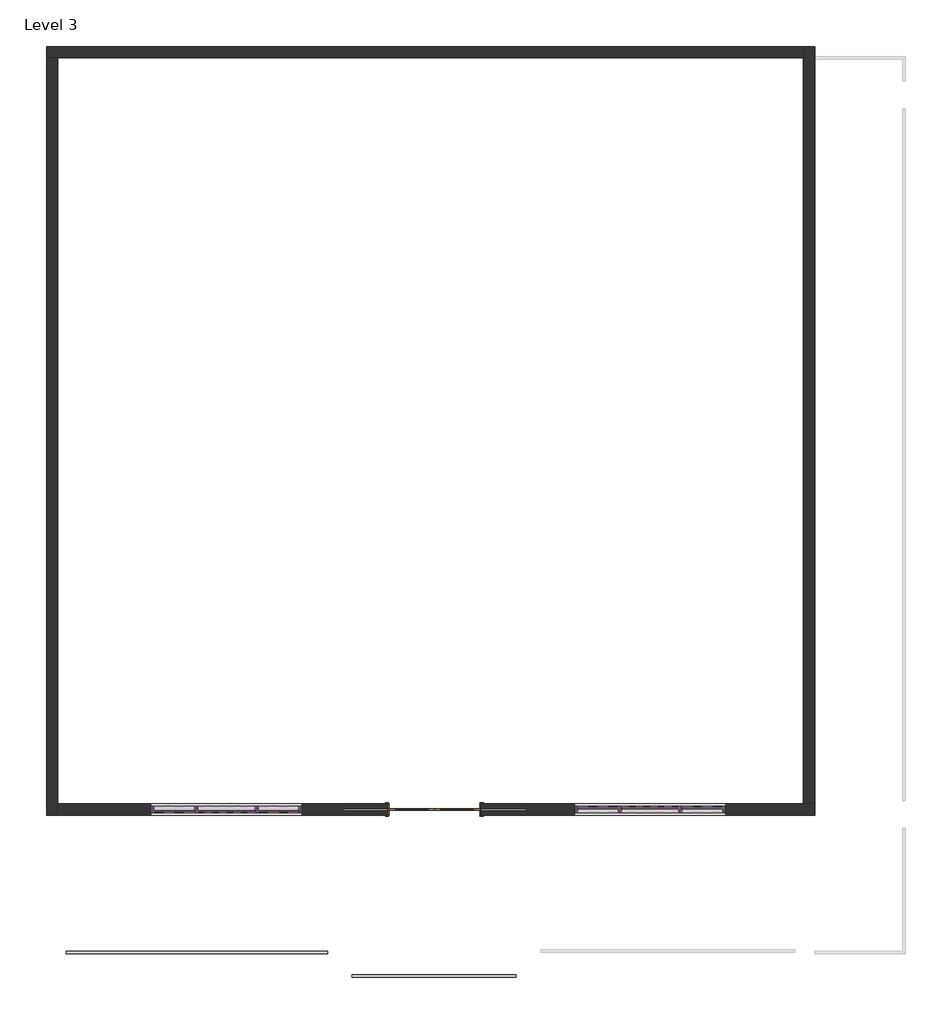
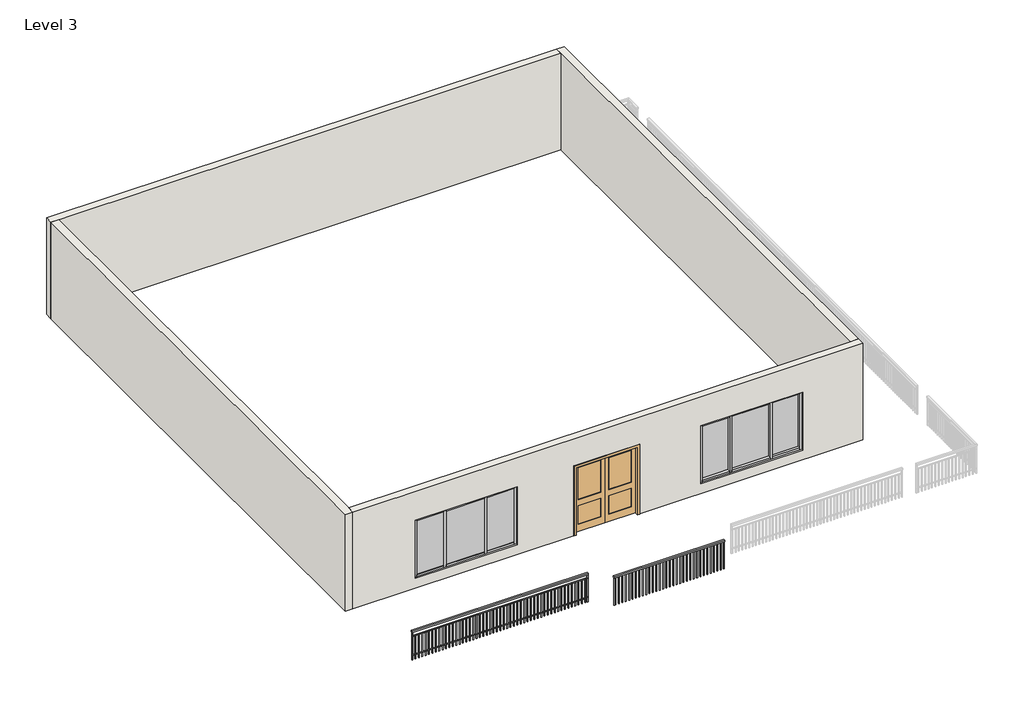
# One storey, part 1 of 4: 20 members, 6 plates, 4 walls, 2 railings, 1 door.
"""IFC4 building model written with IfcOpenShell, lengths in millimetres."""

from ifc_helpers import new_model, si_unit, point, frame, frame_2d, origin, place, context, project, spatial, polyline, circle_curve, trimmed, segment, composite_curve, outline, extrude, faceted_brep, transform, mapped, element, save
from components import door_c75fb906, member_c17f1be2, member_d7472725, member_d60e8053, member_2fae0574, system_panel_glazed_0f3f94b3, system_panel_glazed_6bf442e5

model = new_model("IFC4")

# Units and contexts
model_context = context("Model", 3, world=origin())
ifc_project = project(units=[si_unit("LENGTHUNIT", "METRE", prefix="MILLI")], contexts=[model_context])

# Site, building, storey
site = spatial("IfcSite", under=ifc_project)
building = spatial("IfcBuilding", under=site)
storey = spatial("IfcBuildingStorey", under=building, Name="Level 3", Elevation=3810.0)

# Door
placement = place(None, origin())
door_shape = door_c75fb906(model_context)
element("IfcDoor", 1, ObjectType="Door-Interior-Double-Pocket-2_Panel-Wood : 72\" x 84\"", at=placement, inside=storey, context=model_context, shape_type="MappedRepresentation", body=[
    mapped(door_shape, transform((-962.0249265, -5957.4949916, 3810.0), x_axis=(-1.0, 0.0, 0.0), y_axis=(0.0, -1.0, 0.0), z_axis=(0.0, 0.0, 1.0))),
])

# Members
member_shape = member_c17f1be2(model_context)
element("IfcMember", 2, ObjectType="Rectangular Mullion : 2.5\" x 5\" rectangular", at=placement, inside=storey, context=model_context, shape_type="MappedRepresentation", body=[
    mapped(member_shape, transform((-6613.5249265, -5957.4949916, 5943.6), x_axis=(0.0, 0.0, 1.0), y_axis=(0.0, 1.0, 0.0), z_axis=(-1.0, 0.0, 0.0))),
])
element("IfcMember", 3, ObjectType="Rectangular Mullion : 2.5\" x 5\" rectangular", at=placement, inside=storey, context=model_context, shape_type="MappedRepresentation", body=[
    mapped(member_shape, transform((-4511.6749265, -5957.4949916, 5943.6), x_axis=(0.0, 0.0, 1.0), y_axis=(0.0, 1.0, 0.0), z_axis=(-1.0, 0.0, 0.0))),
])
element("IfcMember", 4, ObjectType="Rectangular Mullion : 2.5\" x 5\" rectangular", at=placement, inside=storey, context=model_context, shape_type="MappedRepresentation", body=[
    mapped(member_shape, transform((4841.8750735, -5957.4949916, 5943.6), x_axis=(0.0, 0.0, 1.0), y_axis=(0.0, -1.0, 0.0), z_axis=(1.0, 0.0, 0.0))),
])
element("IfcMember", 5, ObjectType="Rectangular Mullion : 2.5\" x 5\" rectangular", at=placement, inside=storey, context=model_context, shape_type="MappedRepresentation", body=[
    mapped(member_shape, transform((2740.0250735, -5957.4949916, 5943.6), x_axis=(0.0, 0.0, 1.0), y_axis=(0.0, -1.0, 0.0), z_axis=(1.0, 0.0, 0.0))),
])
element("IfcMember", 6, ObjectType="Rectangular Mullion : 2.5\" x 5\" rectangular", at=placement, inside=storey, context=model_context, shape_type="MappedRepresentation", body=[
    mapped(member_shape, transform((-3692.5249265, -5957.4949916, 4114.8), x_axis=(0.0, 0.0, -1.0), y_axis=(0.0, 1.0, 0.0), z_axis=(1.0, 0.0, 0.0))),
])
element("IfcMember", 7, ObjectType="Rectangular Mullion : 2.5\" x 5\" rectangular", at=placement, inside=storey, context=model_context, shape_type="MappedRepresentation", body=[
    mapped(member_shape, transform((-5794.3749265, -5957.4949916, 4114.8), x_axis=(0.0, 0.0, -1.0), y_axis=(0.0, 1.0, 0.0), z_axis=(1.0, 0.0, 0.0))),
])
element("IfcMember", 8, ObjectType="Rectangular Mullion : 2.5\" x 5\" rectangular", at=placement, inside=storey, context=model_context, shape_type="MappedRepresentation", body=[
    mapped(member_shape, transform((1920.8750735, -5957.4949916, 4114.8), x_axis=(0.0, 0.0, -1.0), y_axis=(0.0, -1.0, 0.0), z_axis=(-1.0, 0.0, 0.0))),
])
element("IfcMember", 9, ObjectType="Rectangular Mullion : 2.5\" x 5\" rectangular", at=placement, inside=storey, context=model_context, shape_type="MappedRepresentation", body=[
    mapped(member_shape, transform((4022.7250735, -5957.4949916, 4114.8), x_axis=(0.0, 0.0, -1.0), y_axis=(0.0, -1.0, 0.0), z_axis=(-1.0, 0.0, 0.0))),
])
member_2_shape = member_d7472725(model_context)
element("IfcMember", 10, ObjectType="Rectangular Mullion : 2.5\" x 5\" rectangular", at=placement, inside=storey, context=model_context, shape_type="MappedRepresentation", body=[
    mapped(member_2_shape, transform((-4575.1749265, -5957.4949916, 4114.8), x_axis=(0.0, 0.0, -1.0), y_axis=(0.0, 1.0, 0.0), z_axis=(1.0, 0.0, 0.0))),
])
element("IfcMember", 11, ObjectType="Rectangular Mullion : 2.5\" x 5\" rectangular", at=placement, inside=storey, context=model_context, shape_type="MappedRepresentation", body=[
    mapped(member_2_shape, transform((2803.5250735, -5957.4949916, 4114.8), x_axis=(0.0, 0.0, -1.0), y_axis=(0.0, -1.0, 0.0), z_axis=(-1.0, 0.0, 0.0))),
])
element("IfcMember", 12, ObjectType="Rectangular Mullion : 2.5\" x 5\" rectangular", at=placement, inside=storey, context=model_context, shape_type="MappedRepresentation", body=[
    mapped(member_2_shape, transform((-5730.8749265, -5957.4949916, 5943.6), x_axis=(0.0, 0.0, 1.0), y_axis=(0.0, 1.0, 0.0), z_axis=(-1.0, 0.0, 0.0))),
])
element("IfcMember", 13, ObjectType="Rectangular Mullion : 2.5\" x 5\" rectangular", at=placement, inside=storey, context=model_context, shape_type="MappedRepresentation", body=[
    mapped(member_2_shape, transform((3959.2250735, -5957.4949916, 5943.6), x_axis=(0.0, 0.0, 1.0), y_axis=(0.0, -1.0, 0.0), z_axis=(1.0, 0.0, 0.0))),
])
member_3_shape = member_d60e8053(model_context)
element("IfcMember", 14, ObjectType="Rectangular Mullion : 2.5\" x 5\" rectangular", at=placement, inside=storey, context=model_context, shape_type="MappedRepresentation", body=[
    mapped(member_3_shape, transform((-5762.6249265, -5957.4949916, 4114.8), x_axis=(-1.0, 0.0, 0.0), y_axis=(0.0, 1.0, 0.0), z_axis=(0.0, 0.0, -1.0))),
])
element("IfcMember", 15, ObjectType="Rectangular Mullion : 2.5\" x 5\" rectangular", at=placement, inside=storey, context=model_context, shape_type="MappedRepresentation", body=[
    mapped(member_3_shape, transform((-4543.4249265, -5957.4949916, 4114.8), x_axis=(-1.0, 0.0, 0.0), y_axis=(0.0, 1.0, 0.0), z_axis=(0.0, 0.0, -1.0))),
])
element("IfcMember", 16, ObjectType="Rectangular Mullion : 2.5\" x 5\" rectangular", at=placement, inside=storey, context=model_context, shape_type="MappedRepresentation", body=[
    mapped(member_3_shape, transform((2771.7750735, -5957.4949916, 4114.8), x_axis=(1.0, 0.0, 0.0), y_axis=(0.0, -1.0, 0.0), z_axis=(0.0, 0.0, -1.0))),
])
element("IfcMember", 17, ObjectType="Rectangular Mullion : 2.5\" x 5\" rectangular", at=placement, inside=storey, context=model_context, shape_type="MappedRepresentation", body=[
    mapped(member_3_shape, transform((3990.9750735, -5957.4949916, 4114.8), x_axis=(1.0, 0.0, 0.0), y_axis=(0.0, -1.0, 0.0), z_axis=(0.0, 0.0, -1.0))),
])
member_4_shape = member_2fae0574(model_context)
element("IfcMember", 18, ObjectType="Rectangular Mullion : 2.5\" x 5\" rectangular", at=placement, inside=storey, context=model_context, shape_type="MappedRepresentation", body=[
    mapped(member_4_shape, transform((-3629.0249265, -5957.4949916, 5943.6), x_axis=(1.0, 0.0, 0.0), y_axis=(0.0, 1.0, 0.0), z_axis=(0.0, 0.0, 1.0))),
])
element("IfcMember", 19, ObjectType="Rectangular Mullion : 2.5\" x 5\" rectangular", at=placement, inside=storey, context=model_context, shape_type="MappedRepresentation", body=[
    mapped(member_4_shape, transform((1857.3750735, -5957.4949916, 5943.6), x_axis=(-1.0, 0.0, 0.0), y_axis=(0.0, -1.0, 0.0), z_axis=(0.0, 0.0, 1.0))),
])
element("IfcMember", 20, ObjectType="Rectangular Mullion : 2.5\" x 5\" rectangular", at=placement, inside=storey, context=model_context, shape_type="MappedRepresentation", body=[
    mapped(member_4_shape, transform((-6677.0249265, -5957.4949916, 4114.8), x_axis=(-1.0, 0.0, 0.0), y_axis=(0.0, 1.0, 0.0), z_axis=(0.0, 0.0, -1.0))),
])
element("IfcMember", 21, ObjectType="Rectangular Mullion : 2.5\" x 5\" rectangular", at=placement, inside=storey, context=model_context, shape_type="MappedRepresentation", body=[
    mapped(member_4_shape, transform((4905.3750735, -5957.4949916, 4114.8), x_axis=(1.0, 0.0, 0.0), y_axis=(0.0, -1.0, 0.0), z_axis=(0.0, 0.0, -1.0))),
])

# Plates
system_panel_glazed_shape = system_panel_glazed_0f3f94b3(model_context)
element("IfcPlate", 22, ObjectType="System Panel : Glazed", at=placement, inside=storey, context=model_context, shape_type="MappedRepresentation", body=[
    mapped(system_panel_glazed_shape, transform((-4102.0999265, -5957.4949916, 4178.3), x_axis=(-1.0, 0.0, 0.0), y_axis=(0.0, -1.0, 0.0), z_axis=(0.0, 0.0, 1.0))),
])
element("IfcPlate", 23, ObjectType="System Panel : Glazed", at=placement, inside=storey, context=model_context, shape_type="MappedRepresentation", body=[
    mapped(system_panel_glazed_shape, transform((2330.4500735, -5957.4949916, 4178.3), x_axis=(1.0, 0.0, 0.0), y_axis=(0.0, 1.0, 0.0), z_axis=(0.0, 0.0, 1.0))),
])
element("IfcPlate", 24, ObjectType="System Panel : Glazed", at=placement, inside=storey, context=model_context, shape_type="MappedRepresentation", body=[
    mapped(system_panel_glazed_shape, transform((-6203.9499265, -5957.4949916, 4178.3), x_axis=(-1.0, 0.0, 0.0), y_axis=(0.0, -1.0, 0.0), z_axis=(0.0, 0.0, 1.0))),
])
element("IfcPlate", 25, ObjectType="System Panel : Glazed", at=placement, inside=storey, context=model_context, shape_type="MappedRepresentation", body=[
    mapped(system_panel_glazed_shape, transform((4432.3000735, -5957.4949916, 4178.3), x_axis=(1.0, 0.0, 0.0), y_axis=(0.0, 1.0, 0.0), z_axis=(0.0, 0.0, 1.0))),
])
system_panel_glazed_2_shape = system_panel_glazed_6bf442e5(model_context)
element("IfcPlate", 26, ObjectType="System Panel : Glazed", at=placement, inside=storey, context=model_context, shape_type="MappedRepresentation", body=[
    mapped(system_panel_glazed_2_shape, transform((-5153.0249265, -5957.4949916, 4178.3), x_axis=(-1.0, 0.0, 0.0), y_axis=(0.0, -1.0, 0.0), z_axis=(0.0, 0.0, 1.0))),
])
element("IfcPlate", 27, ObjectType="System Panel : Glazed", at=placement, inside=storey, context=model_context, shape_type="MappedRepresentation", body=[
    mapped(system_panel_glazed_2_shape, transform((3381.3750735, -5957.4949916, 4178.3), x_axis=(1.0, 0.0, 0.0), y_axis=(0.0, 1.0, 0.0), z_axis=(0.0, 0.0, 1.0))),
])

# Railings
element("IfcRailing", 28, ObjectType="Handrail - Rectangular", at=placement, inside=storey, context=model_context, shape_type="SweptSolid", body=[
    extrude(outline(polyline([(-8376.1341656, -8858.0634361), (-8376.1341656, -8807.2634361), (-3118.3341656, -8807.2634361), (-3118.3341656, -8858.0634361), (-8376.1341656, -8858.0634361)])), frame((0.0, 0.0, 4673.6), z_axis=(0.0, 0.0, 1.0), x_axis=(1.0, 0.0, 0.0)), (0.0, 0.0, 1.0), 50.8),
    extrude(outline(composite_curve([segment(trimmed(circle_curve(frame_2d((-8832.6634361, 4559.3)), 12.7), [point((-8819.9634361, 4559.3))], [point((-8845.3634361, 4559.3))], False, "CARTESIAN"), True, "CONTINUOUS"), segment(trimmed(circle_curve(frame_2d((-8832.6634361, 4559.3)), 12.7), [point((-8845.3634361, 4559.3))], [point((-8819.9634361, 4559.3))], False, "CARTESIAN"), True, "CONTINUOUS")], self_intersect=False)), frame((-8376.1341656, 0.0, 0.0), z_axis=(1.0, 0.0, 0.0), x_axis=(0.0, 1.0, 0.0)), (0.0, 0.0, 1.0), 5257.8),
    extrude(outline(composite_curve([segment(trimmed(circle_curve(frame_2d((-8832.6634361, 3949.7)), 12.7), [point((-8819.9634361, 3949.7))], [point((-8845.3634361, 3949.7))], False, "CARTESIAN"), True, "CONTINUOUS"), segment(trimmed(circle_curve(frame_2d((-8832.6634361, 3949.7)), 12.7), [point((-8845.3634361, 3949.7))], [point((-8819.9634361, 3949.7))], False, "CARTESIAN"), True, "CONTINUOUS")], self_intersect=False)), frame((-8376.1341656, 0.0, 0.0), z_axis=(1.0, 0.0, 0.0), x_axis=(0.0, 1.0, 0.0)), (0.0, 0.0, 1.0), 5257.8),
    extrude(outline(polyline([(-3204.0591656, -8842.1884361), (-3204.0591656, -8823.1384361), (-3185.0091656, -8823.1384361), (-3185.0091656, -8842.1884361), (-3204.0591656, -8842.1884361)])), frame((0.0, 0.0, 3810.0), z_axis=(0.0, 0.0, 1.0), x_axis=(1.0, 0.0, 0.0)), (0.0, 0.0, 1.0), 736.6),
    extrude(outline(polyline([(-3305.6591656, -8842.1884361), (-3305.6591656, -8823.1384361), (-3286.6091656, -8823.1384361), (-3286.6091656, -8842.1884361), (-3305.6591656, -8842.1884361)])), frame((0.0, 0.0, 3810.0), z_axis=(0.0, 0.0, 1.0), x_axis=(1.0, 0.0, 0.0)), (0.0, 0.0, 1.0), 736.6),
    extrude(outline(polyline([(-3407.2591656, -8842.1884361), (-3407.2591656, -8823.1384361), (-3388.2091656, -8823.1384361), (-3388.2091656, -8842.1884361), (-3407.2591656, -8842.1884361)])), frame((0.0, 0.0, 3810.0), z_axis=(0.0, 0.0, 1.0), x_axis=(1.0, 0.0, 0.0)), (0.0, 0.0, 1.0), 736.6),
    extrude(outline(polyline([(-3508.8591656, -8842.1884361), (-3508.8591656, -8823.1384361), (-3489.8091656, -8823.1384361), (-3489.8091656, -8842.1884361), (-3508.8591656, -8842.1884361)])), frame((0.0, 0.0, 3810.0), z_axis=(0.0, 0.0, 1.0), x_axis=(1.0, 0.0, 0.0)), (0.0, 0.0, 1.0), 736.6),
    extrude(outline(polyline([(-3610.4591656, -8842.1884361), (-3610.4591656, -8823.1384361), (-3591.4091656, -8823.1384361), (-3591.4091656, -8842.1884361), (-3610.4591656, -8842.1884361)])), frame((0.0, 0.0, 3810.0), z_axis=(0.0, 0.0, 1.0), x_axis=(1.0, 0.0, 0.0)), (0.0, 0.0, 1.0), 736.6),
    extrude(outline(polyline([(-3712.0591656, -8842.1884361), (-3712.0591656, -8823.1384361), (-3693.0091656, -8823.1384361), (-3693.0091656, -8842.1884361), (-3712.0591656, -8842.1884361)])), frame((0.0, 0.0, 3810.0), z_axis=(0.0, 0.0, 1.0), x_axis=(1.0, 0.0, 0.0)), (0.0, 0.0, 1.0), 736.6),
    extrude(outline(polyline([(-3813.6591656, -8842.1884361), (-3813.6591656, -8823.1384361), (-3794.6091656, -8823.1384361), (-3794.6091656, -8842.1884361), (-3813.6591656, -8842.1884361)])), frame((0.0, 0.0, 3810.0), z_axis=(0.0, 0.0, 1.0), x_axis=(1.0, 0.0, 0.0)), (0.0, 0.0, 1.0), 736.6),
    extrude(outline(polyline([(-3915.2591656, -8842.1884361), (-3915.2591656, -8823.1384361), (-3896.2091656, -8823.1384361), (-3896.2091656, -8842.1884361), (-3915.2591656, -8842.1884361)])), frame((0.0, 0.0, 3810.0), z_axis=(0.0, 0.0, 1.0), x_axis=(1.0, 0.0, 0.0)), (0.0, 0.0, 1.0), 736.6),
    extrude(outline(polyline([(-4016.8591656, -8842.1884361), (-4016.8591656, -8823.1384361), (-3997.8091656, -8823.1384361), (-3997.8091656, -8842.1884361), (-4016.8591656, -8842.1884361)])), frame((0.0, 0.0, 3810.0), z_axis=(0.0, 0.0, 1.0), x_axis=(1.0, 0.0, 0.0)), (0.0, 0.0, 1.0), 736.6),
    extrude(outline(polyline([(-4118.4591656, -8842.1884361), (-4118.4591656, -8823.1384361), (-4099.4091656, -8823.1384361), (-4099.4091656, -8842.1884361), (-4118.4591656, -8842.1884361)])), frame((0.0, 0.0, 3810.0), z_axis=(0.0, 0.0, 1.0), x_axis=(1.0, 0.0, 0.0)), (0.0, 0.0, 1.0), 736.6),
    extrude(outline(polyline([(-4220.0591656, -8842.1884361), (-4220.0591656, -8823.1384361), (-4201.0091656, -8823.1384361), (-4201.0091656, -8842.1884361), (-4220.0591656, -8842.1884361)])), frame((0.0, 0.0, 3810.0), z_axis=(0.0, 0.0, 1.0), x_axis=(1.0, 0.0, 0.0)), (0.0, 0.0, 1.0), 736.6),
    extrude(outline(polyline([(-4321.6591656, -8842.1884361), (-4321.6591656, -8823.1384361), (-4302.6091656, -8823.1384361), (-4302.6091656, -8842.1884361), (-4321.6591656, -8842.1884361)])), frame((0.0, 0.0, 3810.0), z_axis=(0.0, 0.0, 1.0), x_axis=(1.0, 0.0, 0.0)), (0.0, 0.0, 1.0), 736.6),
    extrude(outline(polyline([(-4423.2591656, -8842.1884361), (-4423.2591656, -8823.1384361), (-4404.2091656, -8823.1384361), (-4404.2091656, -8842.1884361), (-4423.2591656, -8842.1884361)])), frame((0.0, 0.0, 3810.0), z_axis=(0.0, 0.0, 1.0), x_axis=(1.0, 0.0, 0.0)), (0.0, 0.0, 1.0), 736.6),
    extrude(outline(polyline([(-4524.8591656, -8842.1884361), (-4524.8591656, -8823.1384361), (-4505.8091656, -8823.1384361), (-4505.8091656, -8842.1884361), (-4524.8591656, -8842.1884361)])), frame((0.0, 0.0, 3810.0), z_axis=(0.0, 0.0, 1.0), x_axis=(1.0, 0.0, 0.0)), (0.0, 0.0, 1.0), 736.6),
    extrude(outline(polyline([(-4626.4591656, -8842.1884361), (-4626.4591656, -8823.1384361), (-4607.4091656, -8823.1384361), (-4607.4091656, -8842.1884361), (-4626.4591656, -8842.1884361)])), frame((0.0, 0.0, 3810.0), z_axis=(0.0, 0.0, 1.0), x_axis=(1.0, 0.0, 0.0)), (0.0, 0.0, 1.0), 736.6),
    extrude(outline(polyline([(-4728.0591656, -8842.1884361), (-4728.0591656, -8823.1384361), (-4709.0091656, -8823.1384361), (-4709.0091656, -8842.1884361), (-4728.0591656, -8842.1884361)])), frame((0.0, 0.0, 3810.0), z_axis=(0.0, 0.0, 1.0), x_axis=(1.0, 0.0, 0.0)), (0.0, 0.0, 1.0), 736.6),
    extrude(outline(polyline([(-4829.6591656, -8842.1884361), (-4829.6591656, -8823.1384361), (-4810.6091656, -8823.1384361), (-4810.6091656, -8842.1884361), (-4829.6591656, -8842.1884361)])), frame((0.0, 0.0, 3810.0), z_axis=(0.0, 0.0, 1.0), x_axis=(1.0, 0.0, 0.0)), (0.0, 0.0, 1.0), 736.6),
    extrude(outline(polyline([(-4931.2591656, -8842.1884361), (-4931.2591656, -8823.1384361), (-4912.2091656, -8823.1384361), (-4912.2091656, -8842.1884361), (-4931.2591656, -8842.1884361)])), frame((0.0, 0.0, 3810.0), z_axis=(0.0, 0.0, 1.0), x_axis=(1.0, 0.0, 0.0)), (0.0, 0.0, 1.0), 736.6),
    extrude(outline(polyline([(-5032.8591656, -8842.1884361), (-5032.8591656, -8823.1384361), (-5013.8091656, -8823.1384361), (-5013.8091656, -8842.1884361), (-5032.8591656, -8842.1884361)])), frame((0.0, 0.0, 3810.0), z_axis=(0.0, 0.0, 1.0), x_axis=(1.0, 0.0, 0.0)), (0.0, 0.0, 1.0), 736.6),
    extrude(outline(polyline([(-5134.4591656, -8842.1884361), (-5134.4591656, -8823.1384361), (-5115.4091656, -8823.1384361), (-5115.4091656, -8842.1884361), (-5134.4591656, -8842.1884361)])), frame((0.0, 0.0, 3810.0), z_axis=(0.0, 0.0, 1.0), x_axis=(1.0, 0.0, 0.0)), (0.0, 0.0, 1.0), 736.6),
    extrude(outline(polyline([(-5236.0591656, -8842.1884361), (-5236.0591656, -8823.1384361), (-5217.0091656, -8823.1384361), (-5217.0091656, -8842.1884361), (-5236.0591656, -8842.1884361)])), frame((0.0, 0.0, 3810.0), z_axis=(0.0, 0.0, 1.0), x_axis=(1.0, 0.0, 0.0)), (0.0, 0.0, 1.0), 736.6),
    extrude(outline(polyline([(-5337.6591656, -8842.1884361), (-5337.6591656, -8823.1384361), (-5318.6091656, -8823.1384361), (-5318.6091656, -8842.1884361), (-5337.6591656, -8842.1884361)])), frame((0.0, 0.0, 3810.0), z_axis=(0.0, 0.0, 1.0), x_axis=(1.0, 0.0, 0.0)), (0.0, 0.0, 1.0), 736.6),
    extrude(outline(polyline([(-5439.2591656, -8842.1884361), (-5439.2591656, -8823.1384361), (-5420.2091656, -8823.1384361), (-5420.2091656, -8842.1884361), (-5439.2591656, -8842.1884361)])), frame((0.0, 0.0, 3810.0), z_axis=(0.0, 0.0, 1.0), x_axis=(1.0, 0.0, 0.0)), (0.0, 0.0, 1.0), 736.6),
    extrude(outline(polyline([(-5540.8591656, -8842.1884361), (-5540.8591656, -8823.1384361), (-5521.8091656, -8823.1384361), (-5521.8091656, -8842.1884361), (-5540.8591656, -8842.1884361)])), frame((0.0, 0.0, 3810.0), z_axis=(0.0, 0.0, 1.0), x_axis=(1.0, 0.0, 0.0)), (0.0, 0.0, 1.0), 736.6),
    extrude(outline(polyline([(-5642.4591656, -8842.1884361), (-5642.4591656, -8823.1384361), (-5623.4091656, -8823.1384361), (-5623.4091656, -8842.1884361), (-5642.4591656, -8842.1884361)])), frame((0.0, 0.0, 3810.0), z_axis=(0.0, 0.0, 1.0), x_axis=(1.0, 0.0, 0.0)), (0.0, 0.0, 1.0), 736.6),
    extrude(outline(polyline([(-5744.0591656, -8842.1884361), (-5744.0591656, -8823.1384361), (-5725.0091656, -8823.1384361), (-5725.0091656, -8842.1884361), (-5744.0591656, -8842.1884361)])), frame((0.0, 0.0, 3810.0), z_axis=(0.0, 0.0, 1.0), x_axis=(1.0, 0.0, 0.0)), (0.0, 0.0, 1.0), 736.6),
    extrude(outline(polyline([(-5845.6591656, -8842.1884361), (-5845.6591656, -8823.1384361), (-5826.6091656, -8823.1384361), (-5826.6091656, -8842.1884361), (-5845.6591656, -8842.1884361)])), frame((0.0, 0.0, 3810.0), z_axis=(0.0, 0.0, 1.0), x_axis=(1.0, 0.0, 0.0)), (0.0, 0.0, 1.0), 736.6),
    extrude(outline(polyline([(-5947.2591656, -8842.1884361), (-5947.2591656, -8823.1384361), (-5928.2091656, -8823.1384361), (-5928.2091656, -8842.1884361), (-5947.2591656, -8842.1884361)])), frame((0.0, 0.0, 3810.0), z_axis=(0.0, 0.0, 1.0), x_axis=(1.0, 0.0, 0.0)), (0.0, 0.0, 1.0), 736.6),
    extrude(outline(polyline([(-6048.8591656, -8842.1884361), (-6048.8591656, -8823.1384361), (-6029.8091656, -8823.1384361), (-6029.8091656, -8842.1884361), (-6048.8591656, -8842.1884361)])), frame((0.0, 0.0, 3810.0), z_axis=(0.0, 0.0, 1.0), x_axis=(1.0, 0.0, 0.0)), (0.0, 0.0, 1.0), 736.6),
    extrude(outline(polyline([(-6150.4591656, -8842.1884361), (-6150.4591656, -8823.1384361), (-6131.4091656, -8823.1384361), (-6131.4091656, -8842.1884361), (-6150.4591656, -8842.1884361)])), frame((0.0, 0.0, 3810.0), z_axis=(0.0, 0.0, 1.0), x_axis=(1.0, 0.0, 0.0)), (0.0, 0.0, 1.0), 736.6),
    extrude(outline(polyline([(-6252.0591656, -8842.1884361), (-6252.0591656, -8823.1384361), (-6233.0091656, -8823.1384361), (-6233.0091656, -8842.1884361), (-6252.0591656, -8842.1884361)])), frame((0.0, 0.0, 3810.0), z_axis=(0.0, 0.0, 1.0), x_axis=(1.0, 0.0, 0.0)), (0.0, 0.0, 1.0), 736.6),
    extrude(outline(polyline([(-6353.6591656, -8842.1884361), (-6353.6591656, -8823.1384361), (-6334.6091656, -8823.1384361), (-6334.6091656, -8842.1884361), (-6353.6591656, -8842.1884361)])), frame((0.0, 0.0, 3810.0), z_axis=(0.0, 0.0, 1.0), x_axis=(1.0, 0.0, 0.0)), (0.0, 0.0, 1.0), 736.6),
    extrude(outline(polyline([(-6455.2591656, -8842.1884361), (-6455.2591656, -8823.1384361), (-6436.2091656, -8823.1384361), (-6436.2091656, -8842.1884361), (-6455.2591656, -8842.1884361)])), frame((0.0, 0.0, 3810.0), z_axis=(0.0, 0.0, 1.0), x_axis=(1.0, 0.0, 0.0)), (0.0, 0.0, 1.0), 736.6),
    extrude(outline(polyline([(-6556.8591656, -8842.1884361), (-6556.8591656, -8823.1384361), (-6537.8091656, -8823.1384361), (-6537.8091656, -8842.1884361), (-6556.8591656, -8842.1884361)])), frame((0.0, 0.0, 3810.0), z_axis=(0.0, 0.0, 1.0), x_axis=(1.0, 0.0, 0.0)), (0.0, 0.0, 1.0), 736.6),
    extrude(outline(polyline([(-6658.4591656, -8842.1884361), (-6658.4591656, -8823.1384361), (-6639.4091656, -8823.1384361), (-6639.4091656, -8842.1884361), (-6658.4591656, -8842.1884361)])), frame((0.0, 0.0, 3810.0), z_axis=(0.0, 0.0, 1.0), x_axis=(1.0, 0.0, 0.0)), (0.0, 0.0, 1.0), 736.6),
    extrude(outline(polyline([(-6760.0591656, -8842.1884361), (-6760.0591656, -8823.1384361), (-6741.0091656, -8823.1384361), (-6741.0091656, -8842.1884361), (-6760.0591656, -8842.1884361)])), frame((0.0, 0.0, 3810.0), z_axis=(0.0, 0.0, 1.0), x_axis=(1.0, 0.0, 0.0)), (0.0, 0.0, 1.0), 736.6),
    extrude(outline(polyline([(-6861.6591656, -8842.1884361), (-6861.6591656, -8823.1384361), (-6842.6091656, -8823.1384361), (-6842.6091656, -8842.1884361), (-6861.6591656, -8842.1884361)])), frame((0.0, 0.0, 3810.0), z_axis=(0.0, 0.0, 1.0), x_axis=(1.0, 0.0, 0.0)), (0.0, 0.0, 1.0), 736.6),
    extrude(outline(polyline([(-6963.2591656, -8842.1884361), (-6963.2591656, -8823.1384361), (-6944.2091656, -8823.1384361), (-6944.2091656, -8842.1884361), (-6963.2591656, -8842.1884361)])), frame((0.0, 0.0, 3810.0), z_axis=(0.0, 0.0, 1.0), x_axis=(1.0, 0.0, 0.0)), (0.0, 0.0, 1.0), 736.6),
    extrude(outline(polyline([(-7064.8591656, -8842.1884361), (-7064.8591656, -8823.1384361), (-7045.8091656, -8823.1384361), (-7045.8091656, -8842.1884361), (-7064.8591656, -8842.1884361)])), frame((0.0, 0.0, 3810.0), z_axis=(0.0, 0.0, 1.0), x_axis=(1.0, 0.0, 0.0)), (0.0, 0.0, 1.0), 736.6),
    extrude(outline(polyline([(-7166.4591656, -8842.1884361), (-7166.4591656, -8823.1384361), (-7147.4091656, -8823.1384361), (-7147.4091656, -8842.1884361), (-7166.4591656, -8842.1884361)])), frame((0.0, 0.0, 3810.0), z_axis=(0.0, 0.0, 1.0), x_axis=(1.0, 0.0, 0.0)), (0.0, 0.0, 1.0), 736.6),
    extrude(outline(polyline([(-7268.0591656, -8842.1884361), (-7268.0591656, -8823.1384361), (-7249.0091656, -8823.1384361), (-7249.0091656, -8842.1884361), (-7268.0591656, -8842.1884361)])), frame((0.0, 0.0, 3810.0), z_axis=(0.0, 0.0, 1.0), x_axis=(1.0, 0.0, 0.0)), (0.0, 0.0, 1.0), 736.6),
    extrude(outline(polyline([(-7369.6591656, -8842.1884361), (-7369.6591656, -8823.1384361), (-7350.6091656, -8823.1384361), (-7350.6091656, -8842.1884361), (-7369.6591656, -8842.1884361)])), frame((0.0, 0.0, 3810.0), z_axis=(0.0, 0.0, 1.0), x_axis=(1.0, 0.0, 0.0)), (0.0, 0.0, 1.0), 736.6),
    extrude(outline(polyline([(-7471.2591656, -8842.1884361), (-7471.2591656, -8823.1384361), (-7452.2091656, -8823.1384361), (-7452.2091656, -8842.1884361), (-7471.2591656, -8842.1884361)])), frame((0.0, 0.0, 3810.0), z_axis=(0.0, 0.0, 1.0), x_axis=(1.0, 0.0, 0.0)), (0.0, 0.0, 1.0), 736.6),
    extrude(outline(polyline([(-7572.8591656, -8842.1884361), (-7572.8591656, -8823.1384361), (-7553.8091656, -8823.1384361), (-7553.8091656, -8842.1884361), (-7572.8591656, -8842.1884361)])), frame((0.0, 0.0, 3810.0), z_axis=(0.0, 0.0, 1.0), x_axis=(1.0, 0.0, 0.0)), (0.0, 0.0, 1.0), 736.6),
    extrude(outline(polyline([(-7674.4591656, -8842.1884361), (-7674.4591656, -8823.1384361), (-7655.4091656, -8823.1384361), (-7655.4091656, -8842.1884361), (-7674.4591656, -8842.1884361)])), frame((0.0, 0.0, 3810.0), z_axis=(0.0, 0.0, 1.0), x_axis=(1.0, 0.0, 0.0)), (0.0, 0.0, 1.0), 736.6),
    extrude(outline(polyline([(-7776.0591656, -8842.1884361), (-7776.0591656, -8823.1384361), (-7757.0091656, -8823.1384361), (-7757.0091656, -8842.1884361), (-7776.0591656, -8842.1884361)])), frame((0.0, 0.0, 3810.0), z_axis=(0.0, 0.0, 1.0), x_axis=(1.0, 0.0, 0.0)), (0.0, 0.0, 1.0), 736.6),
    extrude(outline(polyline([(-7877.6591656, -8842.1884361), (-7877.6591656, -8823.1384361), (-7858.6091656, -8823.1384361), (-7858.6091656, -8842.1884361), (-7877.6591656, -8842.1884361)])), frame((0.0, 0.0, 3810.0), z_axis=(0.0, 0.0, 1.0), x_axis=(1.0, 0.0, 0.0)), (0.0, 0.0, 1.0), 736.6),
    extrude(outline(polyline([(-7979.2591656, -8842.1884361), (-7979.2591656, -8823.1384361), (-7960.2091656, -8823.1384361), (-7960.2091656, -8842.1884361), (-7979.2591656, -8842.1884361)])), frame((0.0, 0.0, 3810.0), z_axis=(0.0, 0.0, 1.0), x_axis=(1.0, 0.0, 0.0)), (0.0, 0.0, 1.0), 736.6),
    extrude(outline(polyline([(-8080.8591656, -8842.1884361), (-8080.8591656, -8823.1384361), (-8061.8091656, -8823.1384361), (-8061.8091656, -8842.1884361), (-8080.8591656, -8842.1884361)])), frame((0.0, 0.0, 3810.0), z_axis=(0.0, 0.0, 1.0), x_axis=(1.0, 0.0, 0.0)), (0.0, 0.0, 1.0), 736.6),
    extrude(outline(polyline([(-8182.4591656, -8842.1884361), (-8182.4591656, -8823.1384361), (-8163.4091656, -8823.1384361), (-8163.4091656, -8842.1884361), (-8182.4591656, -8842.1884361)])), frame((0.0, 0.0, 3810.0), z_axis=(0.0, 0.0, 1.0), x_axis=(1.0, 0.0, 0.0)), (0.0, 0.0, 1.0), 736.6),
    extrude(outline(polyline([(-8284.0591656, -8842.1884361), (-8284.0591656, -8823.1384361), (-8265.0091656, -8823.1384361), (-8265.0091656, -8842.1884361), (-8284.0591656, -8842.1884361)])), frame((0.0, 0.0, 3810.0), z_axis=(0.0, 0.0, 1.0), x_axis=(1.0, 0.0, 0.0)), (0.0, 0.0, 1.0), 736.6),
    extrude(outline(polyline([(-3140.5591656, -8845.3634361), (-3140.5591656, -8819.9634361), (-3115.1591656, -8819.9634361), (-3115.1591656, -8845.3634361), (-3140.5591656, -8845.3634361)])), frame((0.0, 0.0, 3810.0), z_axis=(0.0, 0.0, 1.0), x_axis=(1.0, 0.0, 0.0)), (0.0, 0.0, 1.0), 863.6),
    extrude(outline(polyline([(-8379.3091656, -8845.3634361), (-8379.3091656, -8819.9634361), (-8353.9091656, -8819.9634361), (-8353.9091656, -8845.3634361), (-8379.3091656, -8845.3634361)])), frame((0.0, 0.0, 3810.0), z_axis=(0.0, 0.0, 1.0), x_axis=(1.0, 0.0, 0.0)), (0.0, 0.0, 1.0), 863.6),
])
element("IfcRailing", 29, ObjectType="Handrail - Rectangular 2", at=placement, inside=storey, context=model_context, shape_type="SweptSolid", body=[
    extrude(outline(polyline([(682.1408344, -9284.8949916), (682.1408344, -9335.6949916), (-2619.8591656, -9335.6949916), (-2619.8591656, -9284.8949916), (682.1408344, -9284.8949916)])), frame((0.0, 0.0, 4673.6), z_axis=(0.0, 0.0, 1.0), x_axis=(1.0, 0.0, 0.0)), (0.0, 0.0, 1.0), 50.8),
    extrude(outline(polyline([(-2559.5341656, -9300.7699916), (-2559.5341656, -9319.8199916), (-2578.5841656, -9319.8199916), (-2578.5841656, -9300.7699916), (-2559.5341656, -9300.7699916)])), frame((0.0, 0.0, 3810.0), z_axis=(0.0, 0.0, 1.0), x_axis=(1.0, 0.0, 0.0)), (0.0, 0.0, 1.0), 863.6),
    extrude(outline(polyline([(-2457.9341656, -9300.7699916), (-2457.9341656, -9319.8199916), (-2476.9841656, -9319.8199916), (-2476.9841656, -9300.7699916), (-2457.9341656, -9300.7699916)])), frame((0.0, 0.0, 3810.0), z_axis=(0.0, 0.0, 1.0), x_axis=(1.0, 0.0, 0.0)), (0.0, 0.0, 1.0), 863.6),
    extrude(outline(polyline([(-2356.3341656, -9300.7699916), (-2356.3341656, -9319.8199916), (-2375.3841656, -9319.8199916), (-2375.3841656, -9300.7699916), (-2356.3341656, -9300.7699916)])), frame((0.0, 0.0, 3810.0), z_axis=(0.0, 0.0, 1.0), x_axis=(1.0, 0.0, 0.0)), (0.0, 0.0, 1.0), 863.6),
    extrude(outline(polyline([(-2254.7341656, -9300.7699916), (-2254.7341656, -9319.8199916), (-2273.7841656, -9319.8199916), (-2273.7841656, -9300.7699916), (-2254.7341656, -9300.7699916)])), frame((0.0, 0.0, 3810.0), z_axis=(0.0, 0.0, 1.0), x_axis=(1.0, 0.0, 0.0)), (0.0, 0.0, 1.0), 863.6),
    extrude(outline(polyline([(-2153.1341656, -9300.7699916), (-2153.1341656, -9319.8199916), (-2172.1841656, -9319.8199916), (-2172.1841656, -9300.7699916), (-2153.1341656, -9300.7699916)])), frame((0.0, 0.0, 3810.0), z_axis=(0.0, 0.0, 1.0), x_axis=(1.0, 0.0, 0.0)), (0.0, 0.0, 1.0), 863.6),
    extrude(outline(polyline([(-2051.5341656, -9300.7699916), (-2051.5341656, -9319.8199916), (-2070.5841656, -9319.8199916), (-2070.5841656, -9300.7699916), (-2051.5341656, -9300.7699916)])), frame((0.0, 0.0, 3810.0), z_axis=(0.0, 0.0, 1.0), x_axis=(1.0, 0.0, 0.0)), (0.0, 0.0, 1.0), 863.6),
    extrude(outline(polyline([(-1949.9341656, -9300.7699916), (-1949.9341656, -9319.8199916), (-1968.9841656, -9319.8199916), (-1968.9841656, -9300.7699916), (-1949.9341656, -9300.7699916)])), frame((0.0, 0.0, 3810.0), z_axis=(0.0, 0.0, 1.0), x_axis=(1.0, 0.0, 0.0)), (0.0, 0.0, 1.0), 863.6),
    extrude(outline(polyline([(-1848.3341656, -9300.7699916), (-1848.3341656, -9319.8199916), (-1867.3841656, -9319.8199916), (-1867.3841656, -9300.7699916), (-1848.3341656, -9300.7699916)])), frame((0.0, 0.0, 3810.0), z_axis=(0.0, 0.0, 1.0), x_axis=(1.0, 0.0, 0.0)), (0.0, 0.0, 1.0), 863.6),
    extrude(outline(polyline([(-1746.7341656, -9300.7699916), (-1746.7341656, -9319.8199916), (-1765.7841656, -9319.8199916), (-1765.7841656, -9300.7699916), (-1746.7341656, -9300.7699916)])), frame((0.0, 0.0, 3810.0), z_axis=(0.0, 0.0, 1.0), x_axis=(1.0, 0.0, 0.0)), (0.0, 0.0, 1.0), 863.6),
    extrude(outline(polyline([(-1645.1341656, -9300.7699916), (-1645.1341656, -9319.8199916), (-1664.1841656, -9319.8199916), (-1664.1841656, -9300.7699916), (-1645.1341656, -9300.7699916)])), frame((0.0, 0.0, 3810.0), z_axis=(0.0, 0.0, 1.0), x_axis=(1.0, 0.0, 0.0)), (0.0, 0.0, 1.0), 863.6),
    extrude(outline(polyline([(-1543.5341656, -9300.7699916), (-1543.5341656, -9319.8199916), (-1562.5841656, -9319.8199916), (-1562.5841656, -9300.7699916), (-1543.5341656, -9300.7699916)])), frame((0.0, 0.0, 3810.0), z_axis=(0.0, 0.0, 1.0), x_axis=(1.0, 0.0, 0.0)), (0.0, 0.0, 1.0), 863.6),
    extrude(outline(polyline([(-1441.9341656, -9300.7699916), (-1441.9341656, -9319.8199916), (-1460.9841656, -9319.8199916), (-1460.9841656, -9300.7699916), (-1441.9341656, -9300.7699916)])), frame((0.0, 0.0, 3810.0), z_axis=(0.0, 0.0, 1.0), x_axis=(1.0, 0.0, 0.0)), (0.0, 0.0, 1.0), 863.6),
    extrude(outline(polyline([(-1340.3341656, -9300.7699916), (-1340.3341656, -9319.8199916), (-1359.3841656, -9319.8199916), (-1359.3841656, -9300.7699916), (-1340.3341656, -9300.7699916)])), frame((0.0, 0.0, 3810.0), z_axis=(0.0, 0.0, 1.0), x_axis=(1.0, 0.0, 0.0)), (0.0, 0.0, 1.0), 863.6),
    extrude(outline(polyline([(-1238.7341656, -9300.7699916), (-1238.7341656, -9319.8199916), (-1257.7841656, -9319.8199916), (-1257.7841656, -9300.7699916), (-1238.7341656, -9300.7699916)])), frame((0.0, 0.0, 3810.0), z_axis=(0.0, 0.0, 1.0), x_axis=(1.0, 0.0, 0.0)), (0.0, 0.0, 1.0), 863.6),
    extrude(outline(polyline([(-1137.1341656, -9300.7699916), (-1137.1341656, -9319.8199916), (-1156.1841656, -9319.8199916), (-1156.1841656, -9300.7699916), (-1137.1341656, -9300.7699916)])), frame((0.0, 0.0, 3810.0), z_axis=(0.0, 0.0, 1.0), x_axis=(1.0, 0.0, 0.0)), (0.0, 0.0, 1.0), 863.6),
    extrude(outline(polyline([(-1035.5341656, -9300.7699916), (-1035.5341656, -9319.8199916), (-1054.5841656, -9319.8199916), (-1054.5841656, -9300.7699916), (-1035.5341656, -9300.7699916)])), frame((0.0, 0.0, 3810.0), z_axis=(0.0, 0.0, 1.0), x_axis=(1.0, 0.0, 0.0)), (0.0, 0.0, 1.0), 863.6),
    extrude(outline(polyline([(-933.9341656, -9300.7699916), (-933.9341656, -9319.8199916), (-952.9841656, -9319.8199916), (-952.9841656, -9300.7699916), (-933.9341656, -9300.7699916)])), frame((0.0, 0.0, 3810.0), z_axis=(0.0, 0.0, 1.0), x_axis=(1.0, 0.0, 0.0)), (0.0, 0.0, 1.0), 863.6),
    extrude(outline(polyline([(-832.3341656, -9300.7699916), (-832.3341656, -9319.8199916), (-851.3841656, -9319.8199916), (-851.3841656, -9300.7699916), (-832.3341656, -9300.7699916)])), frame((0.0, 0.0, 3810.0), z_axis=(0.0, 0.0, 1.0), x_axis=(1.0, 0.0, 0.0)), (0.0, 0.0, 1.0), 863.6),
    extrude(outline(polyline([(-730.7341656, -9300.7699916), (-730.7341656, -9319.8199916), (-749.7841656, -9319.8199916), (-749.7841656, -9300.7699916), (-730.7341656, -9300.7699916)])), frame((0.0, 0.0, 3810.0), z_axis=(0.0, 0.0, 1.0), x_axis=(1.0, 0.0, 0.0)), (0.0, 0.0, 1.0), 863.6),
    extrude(outline(polyline([(-629.1341656, -9300.7699916), (-629.1341656, -9319.8199916), (-648.1841656, -9319.8199916), (-648.1841656, -9300.7699916), (-629.1341656, -9300.7699916)])), frame((0.0, 0.0, 3810.0), z_axis=(0.0, 0.0, 1.0), x_axis=(1.0, 0.0, 0.0)), (0.0, 0.0, 1.0), 863.6),
    extrude(outline(polyline([(-527.5341656, -9300.7699916), (-527.5341656, -9319.8199916), (-546.5841656, -9319.8199916), (-546.5841656, -9300.7699916), (-527.5341656, -9300.7699916)])), frame((0.0, 0.0, 3810.0), z_axis=(0.0, 0.0, 1.0), x_axis=(1.0, 0.0, 0.0)), (0.0, 0.0, 1.0), 863.6),
    extrude(outline(polyline([(-425.9341656, -9300.7699916), (-425.9341656, -9319.8199916), (-444.9841656, -9319.8199916), (-444.9841656, -9300.7699916), (-425.9341656, -9300.7699916)])), frame((0.0, 0.0, 3810.0), z_axis=(0.0, 0.0, 1.0), x_axis=(1.0, 0.0, 0.0)), (0.0, 0.0, 1.0), 863.6),
    extrude(outline(polyline([(-324.3341656, -9300.7699916), (-324.3341656, -9319.8199916), (-343.3841656, -9319.8199916), (-343.3841656, -9300.7699916), (-324.3341656, -9300.7699916)])), frame((0.0, 0.0, 3810.0), z_axis=(0.0, 0.0, 1.0), x_axis=(1.0, 0.0, 0.0)), (0.0, 0.0, 1.0), 863.6),
    extrude(outline(polyline([(-222.7341656, -9300.7699916), (-222.7341656, -9319.8199916), (-241.7841656, -9319.8199916), (-241.7841656, -9300.7699916), (-222.7341656, -9300.7699916)])), frame((0.0, 0.0, 3810.0), z_axis=(0.0, 0.0, 1.0), x_axis=(1.0, 0.0, 0.0)), (0.0, 0.0, 1.0), 863.6),
    extrude(outline(polyline([(-121.1341656, -9300.7699916), (-121.1341656, -9319.8199916), (-140.1841656, -9319.8199916), (-140.1841656, -9300.7699916), (-121.1341656, -9300.7699916)])), frame((0.0, 0.0, 3810.0), z_axis=(0.0, 0.0, 1.0), x_axis=(1.0, 0.0, 0.0)), (0.0, 0.0, 1.0), 863.6),
    extrude(outline(polyline([(-19.5341656, -9300.7699916), (-19.5341656, -9319.8199916), (-38.5841656, -9319.8199916), (-38.5841656, -9300.7699916), (-19.5341656, -9300.7699916)])), frame((0.0, 0.0, 3810.0), z_axis=(0.0, 0.0, 1.0), x_axis=(1.0, 0.0, 0.0)), (0.0, 0.0, 1.0), 863.6),
    extrude(outline(polyline([(82.0658344, -9300.7699916), (82.0658344, -9319.8199916), (63.0158344, -9319.8199916), (63.0158344, -9300.7699916), (82.0658344, -9300.7699916)])), frame((0.0, 0.0, 3810.0), z_axis=(0.0, 0.0, 1.0), x_axis=(1.0, 0.0, 0.0)), (0.0, 0.0, 1.0), 863.6),
    extrude(outline(polyline([(183.6658344, -9300.7699916), (183.6658344, -9319.8199916), (164.6158344, -9319.8199916), (164.6158344, -9300.7699916), (183.6658344, -9300.7699916)])), frame((0.0, 0.0, 3810.0), z_axis=(0.0, 0.0, 1.0), x_axis=(1.0, 0.0, 0.0)), (0.0, 0.0, 1.0), 863.6),
    extrude(outline(polyline([(285.2658344, -9300.7699916), (285.2658344, -9319.8199916), (266.2158344, -9319.8199916), (266.2158344, -9300.7699916), (285.2658344, -9300.7699916)])), frame((0.0, 0.0, 3810.0), z_axis=(0.0, 0.0, 1.0), x_axis=(1.0, 0.0, 0.0)), (0.0, 0.0, 1.0), 863.6),
    extrude(outline(polyline([(386.8658344, -9300.7699916), (386.8658344, -9319.8199916), (367.8158344, -9319.8199916), (367.8158344, -9300.7699916), (386.8658344, -9300.7699916)])), frame((0.0, 0.0, 3810.0), z_axis=(0.0, 0.0, 1.0), x_axis=(1.0, 0.0, 0.0)), (0.0, 0.0, 1.0), 863.6),
    extrude(outline(polyline([(488.4658344, -9300.7699916), (488.4658344, -9319.8199916), (469.4158344, -9319.8199916), (469.4158344, -9300.7699916), (488.4658344, -9300.7699916)])), frame((0.0, 0.0, 3810.0), z_axis=(0.0, 0.0, 1.0), x_axis=(1.0, 0.0, 0.0)), (0.0, 0.0, 1.0), 863.6),
    extrude(outline(polyline([(590.0658344, -9300.7699916), (590.0658344, -9319.8199916), (571.0158344, -9319.8199916), (571.0158344, -9300.7699916), (590.0658344, -9300.7699916)])), frame((0.0, 0.0, 3810.0), z_axis=(0.0, 0.0, 1.0), x_axis=(1.0, 0.0, 0.0)), (0.0, 0.0, 1.0), 863.6),
    extrude(outline(polyline([(-2600.8091656, -9300.7699916), (-2600.8091656, -9319.8199916), (-2619.8591656, -9319.8199916), (-2619.8591656, -9300.7699916), (-2600.8091656, -9300.7699916)])), frame((0.0, 0.0, 3810.0), z_axis=(0.0, 0.0, 1.0), x_axis=(1.0, 0.0, 0.0)), (0.0, 0.0, 1.0), 863.6),
    extrude(outline(polyline([(682.1408344, -9300.7699916), (682.1408344, -9319.8199916), (663.0908344, -9319.8199916), (663.0908344, -9300.7699916), (682.1408344, -9300.7699916)])), frame((0.0, 0.0, 3810.0), z_axis=(0.0, 0.0, 1.0), x_axis=(1.0, 0.0, 0.0)), (0.0, 0.0, 1.0), 863.6),
])

# Walls
element("IfcWall", 30, ObjectType="9\" wall", at=placement, inside=storey, context=model_context, shape_type="Brep", body=[
    faceted_brep([(-8772.5249265, 9168.2050084, 3810.0), (-8543.9249265, 9168.2050084, 3810.0), (6467.4750735, 9168.2050084, 3810.0), (6467.4750735, 9168.2050084, 6858.0), (-8543.9249265, 9168.2050084, 6858.0), (-8772.5249265, 9168.2050084, 6858.0), (-8772.5249265, 9396.8050084, 3810.0), (-8772.5249265, 9396.8050084, 6858.0), (6467.4750735, 9396.8050084, 6858.0), (6467.4750735, 9396.8050084, 3810.0)], [[[0, 1, 2, 3, 4, 5]], [[6, 7, 8, 9]], [[2, 1, 0, 6, 9]], [[5, 4, 3, 8, 7]], [[0, 5, 7, 6]], [[3, 2, 9, 8]]]),
])
element("IfcWall", 31, ObjectType="9\" wall", at=placement, inside=storey, context=model_context, shape_type="Brep", body=[
    faceted_brep([(-8543.9249265, -6071.7949916, 3810.0), (-8543.9249265, -5843.1949916, 3810.0), (-8543.9249265, 9168.2050084, 3810.0), (-8543.9249265, 9168.2050084, 6858.0), (-8543.9249265, -5843.1949916, 6858.0), (-8543.9249265, -6071.7949916, 6858.0), (-8772.5249265, -6071.7949916, 3810.0), (-8772.5249265, -6071.7949916, 6858.0), (-8772.5249265, 9168.2050084, 6858.0), (-8772.5249265, 9168.2050084, 3810.0)], [[[0, 1, 2, 3, 4, 5]], [[6, 7, 8, 9]], [[2, 1, 0, 6, 9]], [[5, 4, 3, 8, 7]], [[0, 5, 7, 6]], [[3, 2, 9, 8]]]),
])
element("IfcWall", 32, ObjectType="9\" wall", at=placement, inside=storey, context=model_context, shape_type="Brep", body=[
    faceted_brep([(-8543.9249265, -5843.1949916, 6858.0), (6467.4750735, -5843.1949916, 6858.0), (6696.0750735, -5843.1949916, 6858.0), (6696.0750735, -5843.1949916, 3810.0), (6467.4750735, -5843.1949916, 3810.0), (-22.2249265, -5843.1949916, 3810.0), (-22.2249265, -5843.1949916, 5969.0), (-1901.8249265, -5843.1949916, 5969.0), (-1901.8249265, -5843.1949916, 3810.0), (-8543.9249265, -5843.1949916, 3810.0), (1857.3750735, -5843.1949916, 5943.6), (1857.3750735, -5843.1949916, 4114.8), (4905.3750735, -5843.1949916, 4114.8), (4905.3750735, -5843.1949916, 5943.6), (-3629.0249265, -5843.1949916, 4114.8), (-3629.0249265, -5843.1949916, 5943.6), (-6677.0249265, -5843.1949916, 5943.6), (-6677.0249265, -5843.1949916, 4114.8), (6696.0750735, -6071.7949916, 6858.0), (-8543.9249265, -6071.7949916, 6858.0), (-8543.9249265, -6071.7949916, 3810.0), (-1901.8249265, -6071.7949916, 3810.0), (-1901.8249265, -6071.7949916, 5969.0), (-22.2249265, -6071.7949916, 5969.0), (-22.2249265, -6071.7949916, 3810.0), (6696.0750735, -6071.7949916, 3810.0), (1857.3750735, -6071.7949916, 4114.8), (1857.3750735, -6071.7949916, 5943.6), (4905.3750735, -6071.7949916, 5943.6), (4905.3750735, -6071.7949916, 4114.8), (-3629.0249265, -6071.7949916, 5943.6), (-3629.0249265, -6071.7949916, 4114.8), (-6677.0249265, -6071.7949916, 4114.8), (-6677.0249265, -6071.7949916, 5943.6), (-22.2249265, -5978.1324916, 3810.0), (892.1750735, -5978.1324916, 3810.0), (892.1750735, -5936.8574916, 3810.0), (-22.2249265, -5936.8574916, 3810.0), (-1901.8249265, -5936.8574916, 3810.0), (-2816.2249265, -5936.8574916, 3810.0), (-2816.2249265, -5978.1324916, 3810.0), (-1901.8249265, -5978.1324916, 3810.0), (-2816.2249265, -5978.1324916, 5969.0), (-2816.2249265, -5936.8574916, 5969.0), (-1901.8249265, -5936.8574916, 5969.0), (-22.2249265, -5936.8574916, 5969.0), (892.1750735, -5936.8574916, 5969.0), (892.1750735, -5978.1324916, 5969.0), (-22.2249265, -5978.1324916, 5969.0), (-1901.8249265, -5978.1324916, 5969.0)], [[[0, 1, 2, 3, 4, 5, 6, 7, 8, 9], [10, 11, 12, 13], [14, 15, 16, 17]], [[18, 19, 20, 21, 22, 23, 24, 25], [26, 27, 28, 29], [30, 31, 32, 33]], [[3, 25, 24, 34, 35, 36, 37, 5, 4]], [[20, 9, 8, 38, 39, 40, 41, 21]], [[2, 1, 0, 19, 18]], [[3, 2, 18, 25]], [[0, 9, 20, 19]], [[42, 43, 44, 7, 6, 45, 46, 47, 48, 23, 22, 49]], [[42, 49, 41, 40]], [[49, 22, 21, 41]], [[23, 48, 34, 24]], [[48, 47, 35, 34]], [[47, 46, 36, 35]], [[46, 45, 37, 36]], [[45, 6, 5, 37]], [[7, 44, 38, 8]], [[44, 43, 39, 38]], [[43, 42, 40, 39]], [[10, 27, 26, 11]], [[27, 10, 13, 28]], [[28, 13, 12, 29]], [[11, 26, 29, 12]], [[14, 31, 30, 15]], [[15, 30, 33, 16]], [[16, 33, 32, 17]], [[31, 14, 17, 32]]]),
])
element("IfcWall", 33, ObjectType="9\" wall", at=placement, inside=storey, context=model_context, shape_type="Brep", body=[
    faceted_brep([(6467.4750735, 9396.8050084, 3810.0), (6467.4750735, 9168.2050084, 3810.0), (6467.4750735, -5843.1949916, 3810.0), (6467.4750735, -5843.1949916, 6858.0), (6467.4750735, 9168.2050084, 6858.0), (6467.4750735, 9396.8050084, 6858.0), (6696.0750735, 9396.8050084, 3810.0), (6696.0750735, 9396.8050084, 6858.0), (6696.0750735, -5843.1949916, 6858.0), (6696.0750735, -5843.1949916, 3810.0)], [[[0, 1, 2, 3, 4, 5]], [[6, 7, 8, 9]], [[2, 1, 0, 6, 9]], [[5, 4, 3, 8, 7]], [[0, 5, 7, 6]], [[3, 2, 9, 8]]]),
])

save(model, "model.ifc")

# Revit data of these elements
# Type "Door-Interior-Double-Pocket-2_Panel-Wood : 72\" x 84\""
#   Type Mark = "8"
#   Assembly Code = "C1020300"
#   Analytic Construction = "Wooden"
#   Top Rail = 0' - 4 11/16"
#   Thickness = 0' - 1 3/8"
#   Thermal Resistance (R) = 2.5876 (h·ft²·°F)/BTU
#   Stiles = 0' - 4 3/4"
#   Rough Width = 12' - 2"
#   Rough Height = 7' - 4 1/2"
#   Panel Width = 3' - 0"
#   Lock Rail = 0' - 7 1/2"
#   Location [instance default] = 3' - 1"
#   Height = 7' - 0"
#   Width = 6' - 0"
#   Heat Transfer Coefficient (U) = 0.3865 BTU/(h·ft²·°F)
#   Bottom Rail = 0' - 9 1/8"
#   Panel Open [instance default] = no
#   Trim Material = Cherry
#   Panel Material = door wood colour
#   Frame Material = door wood colour
#   Visual Light Transmittance = 0
#   Solar Heat Gain Coefficient = 0
#   Wall Closure = (empty or 0)
#   Function = (empty or 0)
# Type "Rectangular Mullion : 2.5\" x 5\" rectangular"
#   built-in parameter 1007304 = 0.416667 (stored number, unit not read)
#   built-in parameter 1007301 = 0.104167 (stored number, unit not read)
#   built-in parameter 1007300 = 0.104167 (stored number, unit not read)
# Type "System Panel : Glazed"
#   Construction Type Id = "GSP4R"
#   Analytic Construction = "1/8 in Pilkington single glazing"
#   Visual Light Transmittance = 0.9
#   Solar Heat Gain Coefficient = 0.86
#   Heat Transfer Coefficient (U) = 1.18115 BTU/(h·ft²·°F)
#   Define Thermal Properties by = 1
# Type "Handrail - Rectangular"
#   Assembly Code = "C2010400"
#   built-in parameter 1008612 = 0.0416667 (stored number, unit not read)
#   built-in parameter 1008611 = 0.0416667 (stored number, unit not read)
#   built-in parameter 1008609 = 0.333333 (stored number, unit not read)
#   built-in parameter 1008604 = 0.166667 (stored number, unit not read)
#   built-in parameter 1008603 = 0.166667 (stored number, unit not read)
#   Railing Height = 3' - 0"
#   built-in parameter 1008630 = 2
#   built-in parameter 1008610 = 2
#   built-in parameter 1008618 = Baluster - Square : 3/4"
# Type "Handrail - Rectangular 2"
#   Assembly Code = "C2010400"
#   built-in parameter 1008612 = 0.0416667 (stored number, unit not read)
#   built-in parameter 1008611 = 0.0416667 (stored number, unit not read)
#   built-in parameter 1008609 = 0.333333 (stored number, unit not read)
#   built-in parameter 1008604 = 0.166667 (stored number, unit not read)
#   built-in parameter 1008603 = 0.166667 (stored number, unit not read)
#   Railing Height = 3' - 0"
#   built-in parameter 1008630 = 2
#   built-in parameter 1008610 = 2
#   built-in parameter 1008618 = Baluster - Square : 3/4"
# Type "9\" wall"
#   Assembly Code = "B2010"
#   Layers, outside or top first: 0' - 9" "Laminate, Ivory, Matte" (function 1)
# Element 1 (IfcDoor, "Door-Interior-Double-Pocket-2_Panel-Wood : 72\" x 84\"")
#   Location = 3' - 1"
#   Panel Open = no
#   Phase Created = New Construction
#   Materials on its faces: "door wood colour", "Cherry"
# Elements 2, 3, 4, 5, 6, 7, 8, 9, 10, 11, 12, 13, 14, 15, 16, 17, 18, 19, 20, 21 (IfcMember, "Rectangular Mullion : 2.5\" x 5\" rectangular")
#   Phase Created = New Construction
# Elements 22, 23, 24, 25, 26, 27 (IfcPlate, "System Panel : Glazed")
#   Phase Created = New Construction
#   Materials on its faces: "Glass"
# Element 28 (IfcRailing, "Handrail - Rectangular")
#   Phase Created = New Construction
# Element 29 (IfcRailing, "Handrail - Rectangular 2")
#   Phase Created = New Construction
# Elements 30, 31, 32, 33 (IfcWall, "9\" wall")
#   Top Offset = 0' - 0"
#   Base Offset = 0' - 0"
#   wall height = 10' - 0"
#   Phase Created = New Construction
#   Base Constraint = Level 3
#   Top Constraint = Level 4
#   Materials on its faces: "Laminate, Ivory, Matte"
# Materials
#   "Cherry": class "Wood", colour RGB 226 177 128, transparency 0, Description = "Prunus Serotina", Cost = 0
#   "door wood colour": class "Generic", colour RGB 120 120 120, transparency 0, Cost = 0
#   "Laminate, Ivory, Matte": class "Plastic", colour RGB 247 247 239, transparency 0, Description = "Plastic Laminate - Ivory, Matte", Cost = 0
#   "Glass": class "Glass", colour RGB 0 128 192, transparency 0.75, Description = "Soda Lime Glass", Cost = 0
